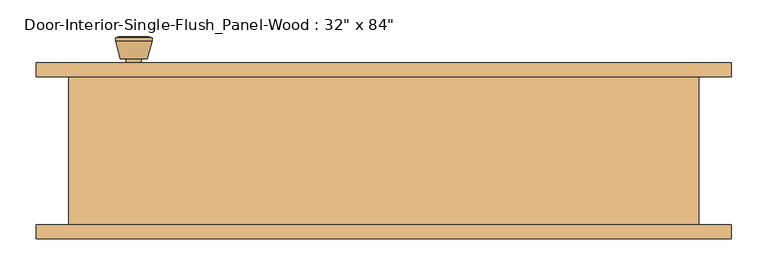
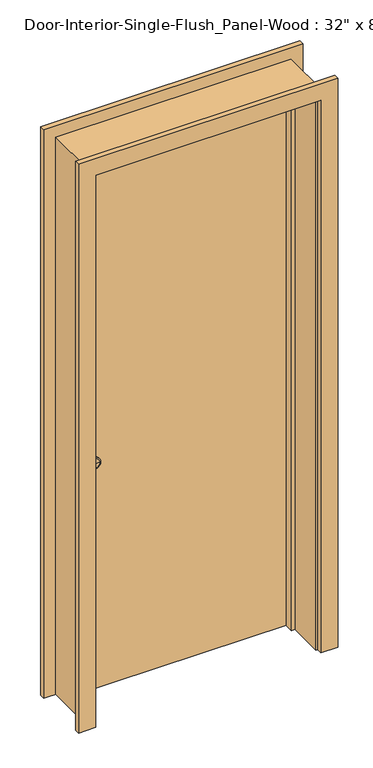
"""IFC4 building model written with IfcOpenShell, lengths in millimetres: door geometry."""

from ifc_helpers import new_model, si_unit, point, frame, frame_2d, origin, origin_with_axes, place, context, project, spatial, polyline, circle_curve, trimmed, segment, composite_curve, outline, extrude, faceted_brep, source, transform, mapped, element, save
from ifc_brep_helpers import plane_surface, cylinder_surface, revolved_surface, advanced_brep


def door_e4576485(model_context):
    return source(origin(), model_context, "Body", "SolidModel", [
        advanced_brep(
        [(-342.9, 57.5, 914.4), (-332.9, 57.5, 914.4), (-352.9, 57.5, 914.4), (-322.4241324, 8.5, 914.4), (-342.9, 8.5, 914.4), (-363.3758676, 8.5, 914.4), (-317.9, 10.3278681, 914.4), (-367.9, 10.3278681, 914.4), (-317.9, 13.7915463, 914.4), (-367.9, 13.7915463, 914.4), (-324.263764, 38.5, 914.4), (-361.536236, 38.5, 914.4), (-332.9, 38.5, 914.4), (-352.9, 38.5, 914.4)],
        [
            (0, 1),
            (1, 2, circle_curve(frame((-342.9, 57.5, 914.4), z_axis=(0.0, 1.0, 0.0), x_axis=(-1.0, 0.0, 0.0)), 10.0)),
            (2, 0),
            (2, 1, circle_curve(frame((-342.9, 57.5, 914.4), z_axis=(0.0, 1.0, 0.0), x_axis=(-1.0, 0.0, 0.0)), 10.0)),
            (3, 4),
            (4, 5),
            (5, 3, circle_curve(frame((-342.9, 8.5, 914.4), z_axis=(0.0, -1.0, 0.0), x_axis=(-1.0, 0.0, 0.0)), 20.4758676)),
            (3, 5, circle_curve(frame((-342.9, 8.5, 914.4), z_axis=(0.0, -1.0, 0.0), x_axis=(-1.0, 0.0, 0.0)), 20.4758676)),
            (6, 3),
            (5, 7),
            (7, 6, circle_curve(frame((-342.9, 10.3278681, 914.4), z_axis=(0.0, -1.0, 0.0), x_axis=(-1.0, 0.0, 0.0)), 25.0)),
            (6, 7, circle_curve(frame((-342.9, 10.3278681, 914.4), z_axis=(0.0, -1.0, 0.0), x_axis=(-1.0, 0.0, 0.0)), 25.0)),
            (8, 6),
            (7, 9),
            (9, 8, circle_curve(frame((-342.9, 13.7915463, 914.4), z_axis=(0.0, -1.0, 0.0), x_axis=(-1.0, 0.0, 0.0)), 25.0)),
            (8, 9, circle_curve(frame((-342.9, 13.7915463, 914.4), z_axis=(0.0, -1.0, 0.0), x_axis=(-1.0, 0.0, 0.0)), 25.0)),
            (10, 8),
            (9, 11),
            (11, 10, circle_curve(frame((-342.9, 38.5, 914.4), z_axis=(0.0, -1.0, 0.0), x_axis=(-1.0, 0.0, 0.0)), 18.636236)),
            (10, 11, circle_curve(frame((-342.9, 38.5, 914.4), z_axis=(0.0, -1.0, 0.0), x_axis=(-1.0, 0.0, 0.0)), 18.636236)),
            (12, 10),
            (11, 13),
            (13, 12, circle_curve(frame((-342.9, 38.5, 914.4), z_axis=(0.0, -1.0, 0.0), x_axis=(-1.0, 0.0, 0.0)), 10.0)),
            (12, 13, circle_curve(frame((-342.9, 38.5, 914.4), z_axis=(0.0, -1.0, 0.0), x_axis=(-1.0, 0.0, 0.0)), 10.0)),
            (1, 12),
            (13, 2),
        ],
        [
            plane_surface(frame((-342.9, 57.5, 914.4), z_axis=(0.0, 1.0, 0.0), x_axis=(-1.0, 0.0, 0.0))),
            plane_surface(frame((-342.9, 8.5, 914.4), z_axis=(0.0, -1.0, 0.0), x_axis=(-1.0, 0.0, 0.0))),
            revolved_surface(polyline([(-363.3758676, 8.5, 914.4), (-367.9, 10.3278681, 914.4)]), (-342.9, 57.5, 914.4), (0.0, 1.0, 0.0)),
            cylinder_surface(frame((-342.9, 57.5, 914.4), z_axis=(0.0, 1.0, 0.0), x_axis=(-1.0, 0.0, 0.0)), 25.0),
            revolved_surface(polyline([(-367.9, 13.7915463, 914.4), (-361.536236, 38.5, 914.4)]), (-342.9, 57.5, 914.4), (0.0, 1.0, 0.0)),
            plane_surface(frame((-342.9, 38.5, 914.4), z_axis=(0.0, 1.0, 0.0), x_axis=(-1.0, 0.0, 0.0))),
            cylinder_surface(frame((-342.9, 57.5, 914.4), z_axis=(0.0, 1.0, 0.0), x_axis=(-1.0, 0.0, 0.0)), 10.0),
        ],
        [
            (0, [[1, 2, 3]]),
            (0, [[-3, 4, -1]]),
            (1, [[5, 6, 7]]),
            (1, [[-6, -5, 8]]),
            (2, [[9, -7, 10, 11]]),
            (2, [[-10, -8, -9, 12]]),
            (3, [[13, -11, 14, 15]]),
            (3, [[-14, -12, -13, 16]]),
            (4, [[17, -15, 18, 19]]),
            (4, [[-18, -16, -17, 20]]),
            (5, [[21, -19, 22, 23]]),
            (5, [[-22, -20, -21, 24]]),
            (6, [[25, -23, 26, -2]]),
            (6, [[-26, -24, -25, -4]]),
        ],
    ),
        extrude(outline(composite_curve([segment(trimmed(circle_curve(frame_2d((914.4, -342.9)), 30.0), [point((914.4, -372.9))], [point((914.4, -312.9))], False, "CARTESIAN"), True, "CONTINUOUS"), segment(trimmed(circle_curve(frame_2d((914.4, -342.9)), 30.0), [point((914.4, -312.9))], [point((914.4, -372.9))], False, "CARTESIAN"), True, "CONTINUOUS")], self_intersect=False)), frame((0.0, 57.5, 0.0), z_axis=(0.0, 1.0, 0.0), x_axis=(0.0, 0.0, 1.0)), (0.0, 0.0, 1.0), 6.0),
        advanced_brep(
        [(-342.9, 104.425, 914.4), (-352.9, 104.425, 914.4), (-332.9, 104.425, 914.4), (-322.4241324, 153.425, 914.4), (-363.3758676, 153.425, 914.4), (-342.9, 153.425, 914.4), (-317.9, 151.5971319, 914.4), (-367.9, 151.5971319, 914.4), (-317.9, 148.1334537, 914.4), (-367.9, 148.1334537, 914.4), (-324.263764, 123.425, 914.4), (-361.536236, 123.425, 914.4), (-332.9, 123.425, 914.4), (-352.9, 123.425, 914.4)],
        [
            (0, 1),
            (1, 2, circle_curve(frame((-342.9, 104.425, 914.4), z_axis=(0.0, -1.0, 0.0), x_axis=(-1.0, 0.0, 0.0)), 10.0)),
            (2, 0),
            (2, 1, circle_curve(frame((-342.9, 104.425, 914.4), z_axis=(0.0, -1.0, 0.0), x_axis=(-1.0, 0.0, 0.0)), 10.0)),
            (3, 4, circle_curve(frame((-342.9, 153.425, 914.4), z_axis=(0.0, 1.0, 0.0), x_axis=(-1.0, 0.0, 0.0)), 20.4758676)),
            (4, 5),
            (5, 3),
            (4, 3, circle_curve(frame((-342.9, 153.425, 914.4), z_axis=(0.0, 1.0, 0.0), x_axis=(-1.0, 0.0, 0.0)), 20.4758676)),
            (6, 7, circle_curve(frame((-342.9, 151.5971319, 914.4), z_axis=(0.0, 1.0, 0.0), x_axis=(-1.0, 0.0, 0.0)), 25.0)),
            (7, 4),
            (3, 6),
            (7, 6, circle_curve(frame((-342.9, 151.5971319, 914.4), z_axis=(0.0, 1.0, 0.0), x_axis=(-1.0, 0.0, 0.0)), 25.0)),
            (8, 9, circle_curve(frame((-342.9, 148.1334537, 914.4), z_axis=(0.0, 1.0, 0.0), x_axis=(-1.0, 0.0, 0.0)), 25.0)),
            (9, 7),
            (6, 8),
            (9, 8, circle_curve(frame((-342.9, 148.1334537, 914.4), z_axis=(0.0, 1.0, 0.0), x_axis=(-1.0, 0.0, 0.0)), 25.0)),
            (10, 11, circle_curve(frame((-342.9, 123.425, 914.4), z_axis=(0.0, 1.0, 0.0), x_axis=(-1.0, 0.0, 0.0)), 18.636236)),
            (11, 9),
            (8, 10),
            (11, 10, circle_curve(frame((-342.9, 123.425, 914.4), z_axis=(0.0, 1.0, 0.0), x_axis=(-1.0, 0.0, 0.0)), 18.636236)),
            (12, 13, circle_curve(frame((-342.9, 123.425, 914.4), z_axis=(0.0, 1.0, 0.0), x_axis=(-1.0, 0.0, 0.0)), 10.0)),
            (13, 11),
            (10, 12),
            (13, 12, circle_curve(frame((-342.9, 123.425, 914.4), z_axis=(0.0, 1.0, 0.0), x_axis=(-1.0, 0.0, 0.0)), 10.0)),
            (1, 13),
            (12, 2),
        ],
        [
            plane_surface(frame((-342.9, 104.425, 914.4), z_axis=(0.0, -1.0, 0.0), x_axis=(-1.0, 0.0, 0.0))),
            plane_surface(frame((-342.9, 153.425, 914.4), z_axis=(0.0, 1.0, 0.0), x_axis=(-1.0, 0.0, 0.0))),
            revolved_surface(polyline([(-363.3758676, 153.425, 914.4), (-367.9, 151.5971319, 914.4)]), (-342.9, 104.425, 914.4), (0.0, -1.0, 0.0)),
            cylinder_surface(frame((-342.9, 104.425, 914.4), z_axis=(0.0, -1.0, 0.0), x_axis=(-1.0, 0.0, 0.0)), 25.0),
            revolved_surface(polyline([(-367.9, 148.1334537, 914.4), (-361.536236, 123.425, 914.4)]), (-342.9, 104.425, 914.4), (0.0, -1.0, 0.0)),
            plane_surface(frame((-342.9, 123.425, 914.4), z_axis=(0.0, -1.0, 0.0), x_axis=(-1.0, 0.0, 0.0))),
            cylinder_surface(frame((-342.9, 104.425, 914.4), z_axis=(0.0, -1.0, 0.0), x_axis=(-1.0, 0.0, 0.0)), 10.0),
        ],
        [
            (0, [[1, 2, 3]]),
            (0, [[-3, 4, -1]]),
            (1, [[5, 6, 7]]),
            (1, [[8, -7, -6]]),
            (2, [[9, 10, -5, 11]]),
            (2, [[12, -11, -8, -10]]),
            (3, [[13, 14, -9, 15]]),
            (3, [[16, -15, -12, -14]]),
            (4, [[17, 18, -13, 19]]),
            (4, [[20, -19, -16, -18]]),
            (5, [[21, 22, -17, 23]]),
            (5, [[24, -23, -20, -22]]),
            (6, [[-2, 25, -21, 26]]),
            (6, [[-4, -26, -24, -25]]),
        ],
    ),
        extrude(outline(composite_curve([segment(trimmed(circle_curve(frame_2d((914.4, -342.9)), 30.0), [point((914.4, -372.9))], [point((914.4, -312.9))], False, "CARTESIAN"), True, "CONTINUOUS"), segment(trimmed(circle_curve(frame_2d((914.4, -342.9)), 30.0), [point((914.4, -312.9))], [point((914.4, -372.9))], False, "CARTESIAN"), True, "CONTINUOUS")], self_intersect=False)), frame((0.0, 98.425, 0.0), z_axis=(0.0, 1.0, 0.0), x_axis=(0.0, 0.0, 1.0)), (0.0, 0.0, 1.0), 6.0),
        extrude(outline(polyline([(406.4, 63.5), (-406.4, 63.5), (-406.4, 98.425), (406.4, 98.425), (406.4, 63.5)])), origin_with_axes(), (0.0, 0.0, 1.0), 2133.6),
        faceted_brep([(431.8, 98.425, 0.0), (431.8, -104.775, 0.0), (406.4, -104.775, 0.0), (406.4, 28.575, 0.0), (393.7, 28.575, 0.0), (393.7, 63.5, 0.0), (406.4, 63.5, 0.0), (406.4, 98.425, 0.0), (431.8, 98.425, 2159.0), (431.8, -104.775, 2159.0), (-431.8, -104.775, 2159.0), (-431.8, -104.775, 0.0), (-406.4, -104.775, 0.0), (-406.4, -104.775, 2133.6), (406.4, -104.775, 2133.6), (406.4, 28.575, 2133.6), (-406.4, 28.575, 2133.6), (-406.4, 28.575, 0.0), (-393.7, 28.575, 0.0), (-393.7, 28.575, 2120.9), (393.7, 28.575, 2120.9), (393.7, 63.5, 2120.9), (-393.7, 63.5, 2120.9), (-393.7, 63.5, 0.0), (-406.4, 63.5, 0.0), (-406.4, 63.5, 2133.6), (406.4, 63.5, 2133.6), (406.4, 98.425, 2133.6), (-406.4, 98.425, 2133.6), (-406.4, 98.425, 0.0), (-431.8, 98.425, 0.0), (-431.8, 98.425, 2159.0)], [[[0, 1, 2, 3, 4, 5, 6, 7]], [[1, 0, 8, 9]], [[2, 1, 9, 10, 11, 12, 13, 14]], [[3, 2, 14, 15]], [[4, 3, 15, 16, 17, 18, 19, 20]], [[5, 4, 20, 21]], [[6, 5, 21, 22, 23, 24, 25, 26]], [[7, 6, 26, 27]], [[0, 7, 27, 28, 29, 30, 31, 8]], [[9, 8, 31, 10]], [[15, 14, 13, 16]], [[21, 20, 19, 22]], [[27, 26, 25, 28]], [[30, 29, 24, 23, 18, 17, 12, 11]], [[10, 31, 30, 11]], [[16, 13, 12, 17]], [[22, 19, 18, 23]], [[28, 25, 24, 29]]]),
        extrude(outline(polyline([(0.0, 412.75), (0.0, 476.25), (2203.45, 476.25), (2203.45, -476.25), (0.0, -476.25), (0.0, -412.75), (2139.95, -412.75), (2139.95, 412.75), (0.0, 412.75)])), frame((0.0, -123.825, 0.0), z_axis=(0.0, 1.0, 0.0), x_axis=(0.0, 0.0, 1.0)), (0.0, 0.0, 1.0), 19.05),
        extrude(outline(polyline([(0.0, 412.75), (0.0, 476.25), (2203.45, 476.25), (2203.45, -476.25), (0.0, -476.25), (0.0, -412.75), (2139.95, -412.75), (2139.95, 412.75), (0.0, 412.75)])), frame((0.0, 98.425, 0.0), z_axis=(0.0, 1.0, 0.0), x_axis=(0.0, 0.0, 1.0)), (0.0, 0.0, 1.0), 19.05),
    ])


if __name__ == "__main__":
    model = new_model("IFC4")
    model_context = context("Model", 3, world=origin())
    ifc_project = project(units=[si_unit("LENGTHUNIT", "METRE", prefix="MILLI")], contexts=[model_context])
    site = spatial("IfcSite", under=ifc_project)
    building = spatial("IfcBuilding", under=site)
    placement = place(None, origin())
    door_shape = door_e4576485(model_context)
    element("IfcDoor", 1, ObjectType="Door-Interior-Single-Flush_Panel-Wood : 32\" x 84\"", at=placement, inside=building, context=model_context, shape_type="MappedRepresentation", body=[
        mapped(door_shape, transform((0.0, 0.0, 0.0), x_axis=(1.0, 0.0, 0.0), y_axis=(0.0, 1.0, 0.0), z_axis=(0.0, 0.0, 1.0))),
    ])
    save(model, "model.ifc")

# Revit data of these elements
# Type "Door-Interior-Single-Flush_Panel-Wood : 32\" x 84\""
#   Type Mark = "13"
#   Assembly Code = "C1020300"
#   Analytic Construction = "Wooden"
#   Thickness = 0' - 1 3/8"
#   Thermal Resistance (R) = 2.5876 (h·ft²·°F)/BTU
#   Swing Angle [instance default] = 90.00°
#   Rough Width = 2' - 10"
#   Rough Height = 7' - 1"
#   Height = 7' - 0"
#   Width = 2' - 8"
#   Heat Transfer Coefficient (U) = 0.3865 BTU/(h·ft²·°F)
#   Trim Material = Cherry
#   Panel Material = Cherry
#   Frame Material = Cherry
#   Door Handle Material = Aluminum
#   Visual Light Transmittance = 0
#   Solar Heat Gain Coefficient = 0
#   Wall Closure = (empty or 0)
#   Function = (empty or 0)
# Element 1 (IfcDoor, "Door-Interior-Single-Flush_Panel-Wood : 32\" x 84\"")
#   Materials on its faces: "Cherry", "Aluminum"
# Materials
#   "Cherry": class "Wood", colour RGB 226 177 128, transparency 0, Description = "Prunus Serotina", Cost = 0
#   "Aluminum": class "Metal", colour RGB 247 247 247, transparency 0, Description = "Aluminum 6061", Cost = 0
